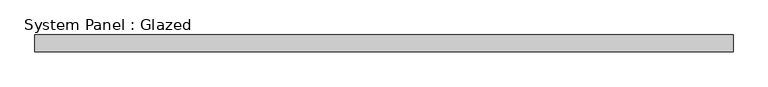
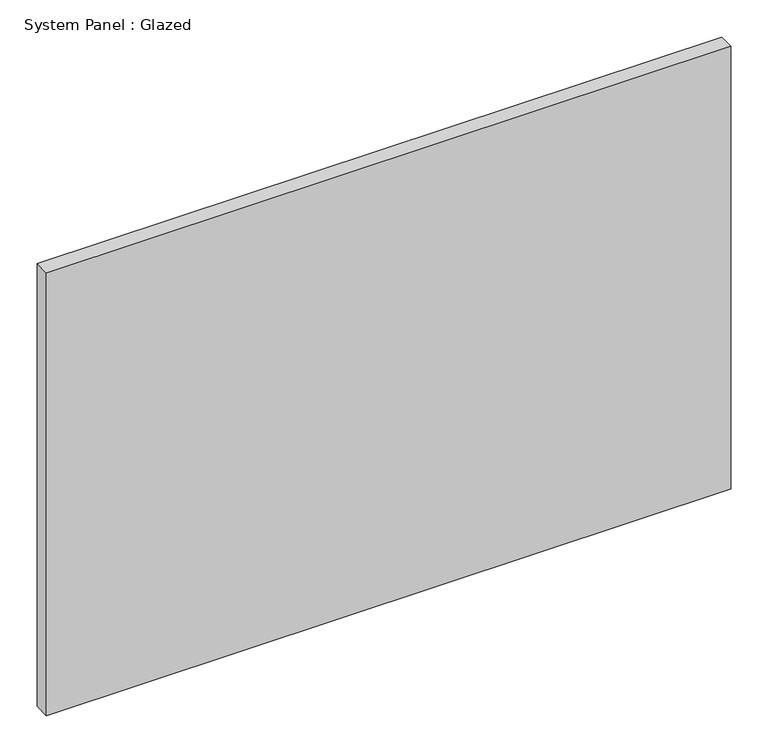
"""IFC4 building model written with IfcOpenShell, lengths in millimetres: plate geometry, System Panel : Glazed."""

from ifc_helpers import new_model, si_unit, origin, origin_with_axes, place, context, project, spatial, polyline, outline, extrude, source, transform, mapped, element, save


def system_panel_glazed_1dd8fbf7(model_context):
    return source(origin(), model_context, "Body", "SweptSolid", [
        extrude(outline(polyline([(533.532314, 19.05), (-533.532314, 19.05), (-533.532314, 44.45), (533.532314, 44.45), (533.532314, 19.05)])), origin_with_axes(), (0.0, 0.0, 1.0), 730.25),
    ])


if __name__ == "__main__":
    model = new_model("IFC4")
    model_context = context("Model", 3, world=origin())
    ifc_project = project(units=[si_unit("LENGTHUNIT", "METRE", prefix="MILLI")], contexts=[model_context])
    site = spatial("IfcSite", under=ifc_project)
    building = spatial("IfcBuilding", under=site)
    placement = place(None, origin())
    system_panel_glazed_shape = system_panel_glazed_1dd8fbf7(model_context)
    element("IfcPlate", 1, ObjectType="System Panel : Glazed", at=placement, inside=building, context=model_context, shape_type="MappedRepresentation", body=[
        mapped(system_panel_glazed_shape, transform((0.0, 0.0, 0.0), x_axis=(1.0, 0.0, 0.0), y_axis=(0.0, 1.0, 0.0), z_axis=(0.0, 0.0, 1.0))),
    ])
    save(model, "model.ifc")

# Revit data of these elements
# Type "System Panel : Glazed"
#   Construction Type Id = "GSP4R"
#   Analytic Construction = "1/8 in Pilkington single glazing"
#   Visual Light Transmittance = 0.9
#   Solar Heat Gain Coefficient = 0.86
#   Heat Transfer Coefficient (U) = 1.18115 BTU/(h·ft²·°F)
#   Define Thermal Properties by = 1
# Element 1 (IfcPlate, "System Panel : Glazed")
#   Materials on its faces: "Glass"
# Materials
#   "Glass": class "Glass", colour RGB 0 128 192, transparency 0.75, Description = "Soda Lime Glass", Cost = 0
